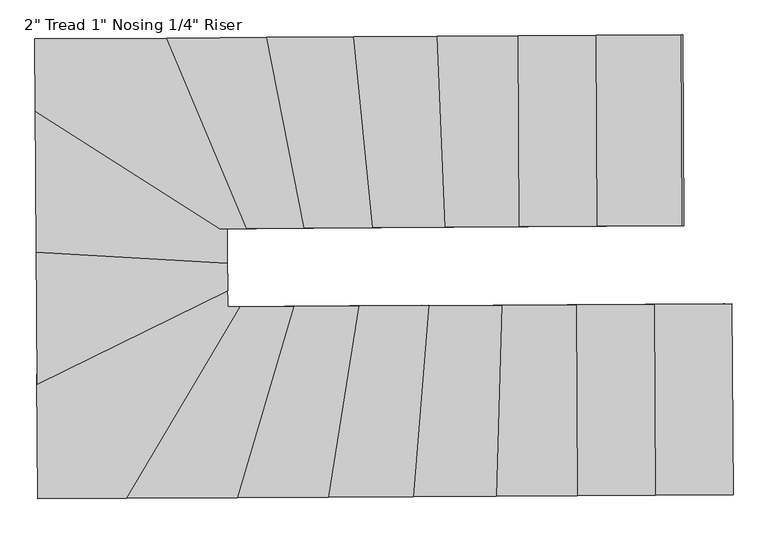
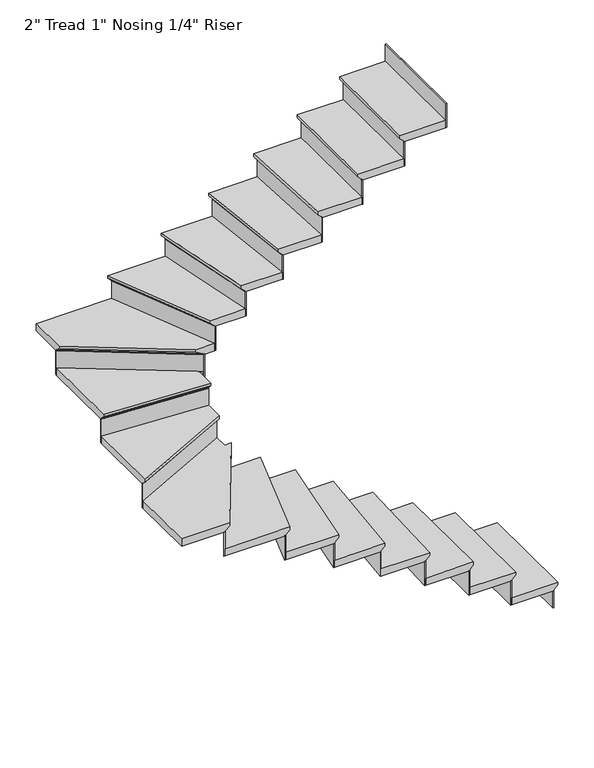
"""IFC4 building model written with IfcOpenShell, lengths in millimetres: stair flight geometry."""

from ifc_helpers import new_model, si_unit, origin, place, context, project, spatial, faceted_brep, source, transform, mapped, element, save


def stair_flight_20cd7bae(model_context):
    return source(origin(), model_context, "Body", "Brep", [
        faceted_brep([(-120.6930289, -3539.621908, 3350.6833333), (-120.6930289, -3539.621908, 3369.7333333), (-116.4891496, -4225.4090232, 3369.7333333), (-116.4891496, -4225.4090232, 3350.6833333), (-146.0925517, -3539.7776072, 3325.2833333), (-141.8886723, -4225.5647224, 3325.2833333), (-425.4873024, -3541.4902988, 3369.7333333), (-421.283423, -4227.277414, 3369.7333333), (-141.8886723, -4225.5647224, 3318.9333333), (-421.283423, -4227.277414, 3318.9333333), (-425.4873024, -3541.4902988, 3318.9333333), (-146.0925517, -3539.7776072, 3318.9333333)], [[[0, 1, 2, 3]], [[4, 0, 3, 5]], [[2, 1, 6, 7]], [[8, 9, 10, 11]], [[2, 7, 9, 8, 5, 3]], [[8, 11, 4, 5]], [[6, 1, 0, 4, 11, 10]], [[7, 6, 10, 9]]]),
        faceted_brep([(-146.0925517, -3539.7776072, 3318.9333333), (-146.0925517, -3539.7776072, 3200.4), (-152.4424324, -3539.816532, 3200.4), (-152.4424324, -3539.816532, 3318.9333333), (-141.8886723, -4225.5647224, 3318.9333333), (-148.238553, -4225.6036472, 3318.9333333), (-148.238553, -4225.6036472, 3200.4), (-141.8886723, -4225.5647224, 3200.4)], [[[0, 1, 2, 3]], [[4, 5, 6, 7]], [[1, 0, 4, 7]], [[2, 1, 7, 6]], [[3, 2, 6, 5]], [[0, 3, 5, 4]]]),
        faceted_brep([(-425.4873024, -3541.4902988, 3488.2666667), (-425.4873024, -3541.4902988, 3318.9333333), (-431.8371831, -3541.5292236, 3318.9333333), (-431.8371831, -3541.5292236, 3488.2666667), (-421.283423, -4227.277414, 3488.2666667), (-427.6333037, -4227.3163388, 3488.2666667), (-427.6333037, -4227.3163388, 3318.9333333), (-421.283423, -4227.277414, 3318.9333333)], [[[0, 1, 2, 3]], [[4, 5, 6, 7]], [[1, 0, 4, 7]], [[2, 1, 7, 6]], [[3, 2, 6, 5]], [[0, 3, 5, 4]]]),
        faceted_brep([(-395.8839002, -4227.1217148, 3539.0666667), (-400.0877796, -3541.3345996, 3539.0666667), (-704.882053, -3543.2029904, 3539.0666667), (-700.6781736, -4228.9901056, 3539.0666667), (-421.283423, -4227.277414, 3488.2666667), (-700.6781736, -4228.9901056, 3488.2666667), (-704.882053, -3543.2029904, 3488.2666667), (-425.4873024, -3541.4902988, 3488.2666667), (-421.283423, -4227.277414, 3494.6166667), (-395.8839002, -4227.1217148, 3520.0166667), (-425.4873024, -3541.4902988, 3494.6166667), (-400.0877796, -3541.3345996, 3520.0166667)], [[[0, 1, 2, 3]], [[4, 5, 6, 7]], [[0, 3, 5, 4, 8, 9]], [[4, 7, 10, 8]], [[2, 1, 11, 10, 7, 6]], [[3, 2, 6, 5]], [[11, 1, 0, 9]], [[10, 11, 9, 8]]]),
        faceted_brep([(-704.882053, -3543.2029904, 3657.6), (-704.882053, -3543.2029904, 3488.2666667), (-711.2319337, -3543.2419152, 3488.2666667), (-711.2319337, -3543.2419152, 3657.6), (-700.6781736, -4228.9901056, 3657.6), (-707.0280543, -4229.0290304, 3657.6), (-707.0280543, -4229.0290304, 3488.2666667), (-700.6781736, -4228.9901056, 3488.2666667)], [[[0, 1, 2, 3]], [[4, 5, 6, 7]], [[1, 0, 4, 7]], [[2, 1, 7, 6]], [[3, 2, 6, 5]], [[0, 3, 5, 4]]]),
        faceted_brep([(-675.2786508, -4228.8344064, 3708.4), (-679.4825302, -3543.0472912, 3708.4), (-971.9344004, -3544.840023, 3708.4), (-992.4483132, -4230.7786584, 3708.4), (-700.6781736, -4228.9901056, 3657.6), (-992.4483132, -4230.7786584, 3657.6), (-971.9344004, -3544.840023, 3657.6), (-704.882053, -3543.2029904, 3657.6), (-700.6781736, -4228.9901056, 3663.95), (-675.2786508, -4228.8344064, 3689.35), (-704.882053, -3543.2029904, 3663.95), (-679.4825302, -3543.0472912, 3689.35)], [[[0, 1, 2, 3]], [[4, 5, 6, 7]], [[0, 3, 5, 4, 8, 9]], [[4, 7, 10, 8]], [[2, 1, 11, 10, 7, 6]], [[3, 2, 6, 5]], [[11, 1, 0, 9]], [[10, 11, 9, 8]]]),
        faceted_brep([(-971.9344004, -3544.840023, 3826.9333333), (-971.9344004, -3544.840023, 3657.6), (-978.2884043, -3544.8789731, 3657.6), (-978.2884043, -3544.8789731, 3826.9333333), (-992.4483132, -4230.7786584, 3826.9333333), (-998.8023171, -4230.8176085, 3826.9333333), (-998.8023171, -4230.8176085, 3657.6), (-992.4483132, -4230.7786584, 3657.6)], [[[0, 1, 2, 3]], [[4, 5, 6, 7]], [[1, 0, 4, 7]], [[2, 1, 7, 6]], [[3, 2, 6, 5]], [[0, 3, 5, 4]]]),
        faceted_brep([(-967.0322975, -4230.6228581, 3877.7333333), (-946.5183848, -3544.6842227, 3877.7333333), (-1233.842238, -3546.4455197, 3877.7333333), (-1289.4900883, -4232.5995264, 3877.7333333), (-992.4483132, -4230.7786584, 3826.9333333), (-1289.4900883, -4232.5995264, 3826.9333333), (-1233.842238, -3546.4455197, 3826.9333333), (-971.9344004, -3544.840023, 3826.9333333), (-992.4483132, -4230.7786584, 3833.2833333), (-967.0322975, -4230.6228581, 3858.6833333), (-971.9344004, -3544.840023, 3833.2833333), (-946.5183848, -3544.6842227, 3858.6833333)], [[[0, 1, 2, 3]], [[4, 5, 6, 7]], [[0, 3, 5, 4, 8, 9]], [[4, 7, 10, 8]], [[2, 1, 11, 10, 7, 6]], [[3, 2, 6, 5]], [[11, 1, 0, 9]], [[10, 11, 9, 8]]]),
        faceted_brep([(-1233.842238, -3546.4455197, 3996.2666667), (-1233.842238, -3546.4455197, 3826.9333333), (-1240.2162558, -3546.4845925, 3826.9333333), (-1240.2162558, -3546.4845925, 3996.2666667), (-1289.4900883, -4232.5995264, 3996.2666667), (-1295.8641061, -4232.6385992, 3996.2666667), (-1295.8641061, -4232.6385992, 3826.9333333), (-1289.4900883, -4232.5995264, 3826.9333333)], [[[0, 1, 2, 3]], [[4, 5, 6, 7]], [[1, 0, 4, 7]], [[2, 1, 7, 6]], [[3, 2, 6, 5]], [[0, 3, 5, 4]]]),
        faceted_brep([(-1263.994017, -4232.4432353, 4047.0666667), (-1208.3461666, -3546.2892286, 4047.0666667), (-1486.5415383, -3547.994568, 4047.0666667), (-1596.081167, -4234.4789317, 4047.0666667), (-1289.4900883, -4232.5995264, 3996.2666667), (-1596.081167, -4234.4789317, 3996.2666667), (-1486.5415383, -3547.994568, 3996.2666667), (-1233.842238, -3546.4455197, 3996.2666667), (-1289.4900883, -4232.5995264, 4002.6166667), (-1263.994017, -4232.4432353, 4028.0166667), (-1233.842238, -3546.4455197, 4002.6166667), (-1208.3461666, -3546.2892286, 4028.0166667)], [[[0, 1, 2, 3]], [[4, 5, 6, 7]], [[0, 3, 5, 4, 8, 9]], [[4, 7, 10, 8]], [[2, 1, 11, 10, 7, 6]], [[3, 2, 6, 5]], [[11, 1, 0, 9]], [[10, 11, 9, 8]]]),
        faceted_brep([(-1486.5415383, -3547.994568, 4165.6), (-1486.5415383, -3547.994568, 3996.2666667), (-1492.9781659, -3548.0340246, 3996.2666667), (-1492.9781659, -3548.0340246, 4165.6), (-1596.081167, -4234.4789317, 4165.6), (-1602.5177946, -4234.5183882, 4165.6), (-1602.5177946, -4234.5183882, 3996.2666667), (-1596.081167, -4234.4789317, 3996.2666667)], [[[0, 1, 2, 3]], [[4, 5, 6, 7]], [[1, 0, 4, 7]], [[2, 1, 7, 6]], [[3, 2, 6, 5]], [[0, 3, 5, 4]]]),
        faceted_brep([(-1570.3346568, -4234.3211054, 4216.4), (-1460.7950281, -3547.8367418, 4216.4), (-1720.1488607, -3549.4265824, 4216.4), (-1922.8306159, -4236.4819079, 4216.4), (-1596.081167, -4234.4789317, 4165.6), (-1922.8306159, -4236.4819079, 4165.6), (-1720.1488607, -3549.4265824, 4165.6), (-1486.5415383, -3547.994568, 4165.6), (-1596.081167, -4234.4789317, 4171.95), (-1570.3346568, -4234.3211054, 4197.35), (-1486.5415383, -3547.994568, 4171.95), (-1460.7950281, -3547.8367418, 4197.35)], [[[0, 1, 2, 3]], [[4, 5, 6, 7]], [[0, 3, 5, 4, 8, 9]], [[4, 7, 10, 8]], [[2, 1, 11, 10, 7, 6]], [[3, 2, 6, 5]], [[11, 1, 0, 9]], [[10, 11, 9, 8]]]),
        faceted_brep([(-1720.1488607, -3549.4265824, 4334.9333333), (-1720.1488607, -3549.4265824, 4165.6), (-1726.781397, -3549.4672399, 4165.6), (-1726.781397, -3549.4672399, 4334.9333333), (-1922.8306159, -4236.4819079, 4334.9333333), (-1929.4631522, -4236.5225654, 4334.9333333), (-1929.4631522, -4236.5225654, 4165.6), (-1922.8306159, -4236.4819079, 4165.6)], [[[0, 1, 2, 3]], [[4, 5, 6, 7]], [[1, 0, 4, 7]], [[2, 1, 7, 6]], [[3, 2, 6, 5]], [[0, 3, 5, 4]]]),
        faceted_brep([(-1896.3004707, -4236.3192779, 4385.7333333), (-1693.6187155, -3549.2639524, 4385.7333333), (-1917.3665941, -3550.6355283, 4385.7333333), (-2324.8688668, -4238.9464049, 4385.7333333), (-1922.8306159, -4236.4819079, 4334.9333333), (-2324.8688668, -4238.9464049, 4334.9333333), (-1917.3665941, -3550.6355283, 4334.9333333), (-1720.1488607, -3549.4265824, 4334.9333333), (-1922.8306159, -4236.4819079, 4341.2833333), (-1896.3004707, -4236.3192779, 4366.6833333), (-1720.1488607, -3549.4265824, 4341.2833333), (-1693.6187155, -3549.2639524, 4366.6833333)], [[[0, 1, 2, 3]], [[4, 5, 6, 7]], [[0, 3, 5, 4, 8, 9]], [[4, 7, 10, 8]], [[2, 1, 11, 10, 7, 6]], [[3, 2, 6, 5]], [[11, 1, 0, 9]], [[10, 11, 9, 8]]]),
        faceted_brep([(-1917.3665941, -3550.6355283, 4504.2666667), (-1917.3665941, -3550.6355283, 4334.9333333), (-1924.7728783, -3550.6809289, 4334.9333333), (-1924.7728783, -3550.6809289, 4504.2666667), (-2324.8688668, -4238.9464049, 4504.2666667), (-2332.275151, -4238.9918055, 4504.2666667), (-2332.275151, -4238.9918055, 4334.9333333), (-2324.8688668, -4238.9464049, 4334.9333333)], [[[0, 1, 2, 3]], [[4, 5, 6, 7]], [[1, 0, 4, 7]], [[2, 1, 7, 6]], [[3, 2, 6, 5]], [[0, 3, 5, 4]]]),
        faceted_brep([(-2615.3480869, -3801.2875551, 4555.0666667), (-2612.6544213, -4240.7105322, 4555.0666667), (-2295.24373, -4238.7648026, 4555.0666667), (-1887.7414574, -3550.4539261, 4555.0666667), (-1931.0711854, -3550.7195376, 4555.0666667), (-1931.5966592, -3464.9979706, 4555.0666667), (-2612.6544213, -4240.7105322, 4504.2666667), (-2615.3480869, -3801.2875551, 4504.2666667), (-1931.5966592, -3464.9979706, 4504.2666667), (-1931.0711854, -3550.7195376, 4504.2666667), (-1917.3665941, -3550.6355283, 4504.2666667), (-2324.8688668, -4238.9464049, 4504.2666667), (-1917.3665941, -3550.6355283, 4510.6166667), (-2324.8688668, -4238.9464049, 4510.6166667), (-1887.7414574, -3550.4539261, 4536.0166667), (-2295.24373, -4238.7648026, 4536.0166667)], [[[0, 1, 2, 3, 4, 5]], [[6, 7, 8, 9, 10, 11]], [[1, 0, 7, 6]], [[11, 10, 12, 13]], [[5, 4, 9, 8]], [[0, 5, 8, 7]], [[14, 3, 2, 15]], [[12, 14, 15, 13]], [[4, 3, 14, 12, 10, 9]], [[2, 1, 6, 11, 13, 15]]]),
        faceted_brep([(-1931.5966592, -3464.9979706, 4673.6), (-1931.5966592, -3464.9979706, 4504.2666667), (-1931.6399076, -3457.9427742, 4504.2666667), (-1931.6399076, -3457.9427742, 4673.6), (-2615.3480869, -3801.2875551, 4673.6), (-2615.3913353, -3794.2323587, 4673.6), (-2615.3913353, -3794.2323587, 4504.2666667), (-2615.3480869, -3801.2875551, 4504.2666667)], [[[0, 1, 2, 3]], [[4, 5, 6, 7]], [[1, 0, 4, 7]], [[2, 1, 7, 6]], [[3, 2, 6, 5]], [[0, 3, 5, 4]]]),
        faceted_brep([(-2615.1750933, -3829.5083406, 4724.4), (-1931.4236656, -3493.2187561, 4724.4), (-1932.1828972, -3369.3638122, 4724.4), (-2618.2387587, -3329.7265819, 4724.4), (-2615.3480869, -3801.2875551, 4673.6), (-2618.2387587, -3329.7265819, 4673.6), (-1932.1828972, -3369.3638122, 4673.6), (-1931.5966592, -3464.9979706, 4673.6), (-2615.3480869, -3801.2875551, 4679.95), (-2615.1750933, -3829.5083406, 4705.35), (-1931.5966592, -3464.9979706, 4679.95), (-1931.4236656, -3493.2187561, 4705.35)], [[[0, 1, 2, 3]], [[4, 5, 6, 7]], [[0, 3, 5, 4, 8, 9]], [[4, 7, 10, 8]], [[2, 1, 11, 10, 7, 6]], [[3, 2, 6, 5]], [[11, 1, 0, 9]], [[10, 11, 9, 8]]]),
        faceted_brep([(-1932.1828972, -3369.3638122, 4842.9333333), (-1932.1828972, -3369.3638122, 4673.6), (-1932.2219015, -3363.0009693, 4673.6), (-1932.2219015, -3363.0009693, 4842.9333333), (-2618.2387587, -3329.7265819, 4842.9333333), (-2618.277763, -3323.363739, 4842.9333333), (-2618.277763, -3323.363739, 4673.6), (-2618.2387587, -3329.7265819, 4673.6)], [[[0, 1, 2, 3]], [[4, 5, 6, 7]], [[1, 0, 4, 7]], [[2, 1, 7, 6]], [[3, 2, 6, 5]], [[0, 3, 5, 4]]]),
        faceted_brep([(-2618.0827416, -3355.1779533, 4893.7333333), (-1932.0268801, -3394.8151835, 4893.7333333), (-1932.783877, -3271.3247869, 4893.7333333), (-1912.0496222, -3271.1976858, 4893.7333333), (-2621.364296, -2819.8515342, 4893.7333333), (-2618.2387587, -3329.7265819, 4842.9333333), (-2621.364296, -2819.8515342, 4842.9333333), (-1912.0496222, -3271.1976858, 4842.9333333), (-1932.783877, -3271.3247869, 4842.9333333), (-1932.1828972, -3369.3638122, 4842.9333333), (-2618.2387587, -3329.7265819, 4849.2833333), (-2618.0827416, -3355.1779533, 4874.6833333), (-1932.1828972, -3369.3638122, 4849.2833333), (-1932.0268801, -3394.8151835, 4874.6833333)], [[[0, 1, 2, 3, 4]], [[5, 6, 7, 8, 9]], [[0, 4, 6, 5, 10, 11]], [[5, 9, 12, 10]], [[2, 1, 13, 12, 9, 8]], [[3, 2, 8, 7]], [[4, 3, 7, 6]], [[13, 1, 0, 11]], [[12, 13, 11, 10]]]),
        faceted_brep([(-1912.0496222, -3271.1976858, 5012.2666667), (-1912.0496222, -3271.1976858, 4842.9333333), (-1900.3341194, -3271.1258697, 4842.9333333), (-1900.3341194, -3271.1258697, 5012.2666667), (-2621.364296, -2819.8515342, 5012.2666667), (-2621.4106144, -2812.2955182, 5012.2666667), (-2621.4106144, -2812.2955182, 4842.9333333), (-2621.364296, -2819.8515342, 4842.9333333)], [[[0, 1, 2, 3]], [[4, 5, 6, 7]], [[1, 0, 4, 7]], [[2, 1, 7, 6]], [[3, 2, 6, 5]], [[0, 3, 5, 4]]]),
        faceted_brep([(-2121.4312205, -2586.6683113, 5063.0666667), (-2622.7748716, -2589.7415511, 5063.0666667), (-2621.1790223, -2850.0755978, 5063.0666667), (-1958.9116334, -3271.4849502, 5063.0666667), (-1835.3232791, -3270.7273529, 5063.0666667), (-2622.7748716, -2589.7415511, 5012.2666667), (-2121.4312205, -2586.6683113, 5012.2666667), (-1835.3232791, -3270.7273529, 5012.2666667), (-1912.0496222, -3271.1976858, 5012.2666667), (-2621.364296, -2819.8515342, 5012.2666667), (-2621.364296, -2819.8515342, 5018.6166667), (-2621.1790223, -2850.0755978, 5044.0166667), (-1912.0496222, -3271.1976858, 5018.6166667), (-1958.9116334, -3271.4849502, 5044.0166667)], [[[0, 1, 2, 3, 4]], [[5, 6, 7, 8, 9]], [[1, 0, 6, 5]], [[2, 1, 5, 9, 10, 11]], [[9, 8, 12, 10]], [[0, 4, 7, 6]], [[13, 3, 2, 11]], [[12, 13, 11, 10]], [[4, 3, 13, 12, 8, 7]]]),
        faceted_brep([(-1835.3232791, -3270.7273529, 5181.6), (-1835.3232791, -3270.7273529, 5012.2666667), (-1828.4578405, -3270.6852677, 5012.2666667), (-1828.4578405, -3270.6852677, 5181.6), (-2121.4312205, -2586.6683113, 5181.6), (-2114.5657819, -2586.6262261, 5181.6), (-2114.5657819, -2586.6262261, 5012.2666667), (-2121.4312205, -2586.6683113, 5012.2666667)], [[[0, 1, 2, 3]], [[4, 5, 6, 7]], [[1, 0, 4, 7]], [[2, 1, 7, 6]], [[3, 2, 6, 5]], [[0, 3, 5, 4]]]),
        faceted_brep([(-2148.8929752, -2586.8366521, 5232.4), (-1862.7850338, -3270.8956936, 5232.4), (-1630.6514822, -3269.4727134, 5232.4), (-1765.0751589, -2584.4838464, 5232.4), (-2121.4312205, -2586.6683113, 5181.6), (-1765.0751589, -2584.4838464, 5181.6), (-1630.6514822, -3269.4727134, 5181.6), (-1835.3232791, -3270.7273529, 5181.6), (-2121.4312205, -2586.6683113, 5187.95), (-2148.8929752, -2586.8366521, 5213.35), (-1835.3232791, -3270.7273529, 5187.95), (-1862.7850338, -3270.8956936, 5213.35)], [[[0, 1, 2, 3]], [[4, 5, 6, 7]], [[0, 3, 5, 4, 8, 9]], [[4, 7, 10, 8]], [[2, 1, 11, 10, 7, 6]], [[3, 2, 6, 5]], [[11, 1, 0, 9]], [[10, 11, 9, 8]]]),
        faceted_brep([(-1630.6514822, -3269.4727134, 5350.9333333), (-1630.6514822, -3269.4727134, 5181.6), (-1624.1881401, -3269.4330931, 5181.6), (-1624.1881401, -3269.4330931, 5350.9333333), (-1765.0751589, -2584.4838464, 5350.9333333), (-1758.6118168, -2584.4442261, 5350.9333333), (-1758.6118168, -2584.4442261, 5181.6), (-1765.0751589, -2584.4838464, 5181.6)], [[[0, 1, 2, 3]], [[4, 5, 6, 7]], [[1, 0, 4, 7]], [[2, 1, 7, 6]], [[3, 2, 6, 5]], [[0, 3, 5, 4]]]),
        faceted_brep([(-1790.9285273, -2584.6423277, 5401.7333333), (-1656.5048506, -3269.6311948, 5401.7333333), (-1385.319119, -3267.9688245, 5401.7333333), (-1452.3132293, -2582.5666138, 5401.7333333), (-1765.0751589, -2584.4838464, 5350.9333333), (-1452.3132293, -2582.5666138, 5350.9333333), (-1385.319119, -3267.9688245, 5350.9333333), (-1630.6514822, -3269.4727134, 5350.9333333), (-1765.0751589, -2584.4838464, 5357.2833333), (-1790.9285273, -2584.6423277, 5382.6833333), (-1630.6514822, -3269.4727134, 5357.2833333), (-1656.5048506, -3269.6311948, 5382.6833333)], [[[0, 1, 2, 3]], [[4, 5, 6, 7]], [[0, 3, 5, 4, 8, 9]], [[4, 7, 10, 8]], [[2, 1, 11, 10, 7, 6]], [[3, 2, 6, 5]], [[11, 1, 0, 9]], [[10, 11, 9, 8]]]),
        faceted_brep([(-1385.319119, -3267.9688245, 5520.2666667), (-1385.319119, -3267.9688245, 5350.9333333), (-1378.942678, -3267.9297369, 5350.9333333), (-1378.942678, -3267.9297369, 5520.2666667), (-1452.3132293, -2582.5666138, 5520.2666667), (-1445.9367882, -2582.5275262, 5520.2666667), (-1445.9367882, -2582.5275262, 5350.9333333), (-1452.3132293, -2582.5666138, 5350.9333333)], [[[0, 1, 2, 3]], [[4, 5, 6, 7]], [[1, 0, 4, 7]], [[2, 1, 7, 6]], [[3, 2, 6, 5]], [[0, 3, 5, 4]]]),
        faceted_brep([(-1477.8189934, -2582.7229643, 5571.0666667), (-1410.8248832, -3268.125175, 5571.0666667), (-1125.1141805, -3266.3737666, 5571.0666667), (-1153.9085026, -2580.7373909, 5571.0666667), (-1452.3132293, -2582.5666138, 5520.2666667), (-1153.9085026, -2580.7373909, 5520.2666667), (-1125.1141805, -3266.3737666, 5520.2666667), (-1385.319119, -3267.9688245, 5520.2666667), (-1452.3132293, -2582.5666138, 5526.6166667), (-1477.8189934, -2582.7229643, 5552.0166667), (-1385.319119, -3267.9688245, 5526.6166667), (-1410.8248832, -3268.125175, 5552.0166667)], [[[0, 1, 2, 3]], [[4, 5, 6, 7]], [[0, 3, 5, 4, 8, 9]], [[4, 7, 10, 8]], [[2, 1, 11, 10, 7, 6]], [[3, 2, 6, 5]], [[11, 1, 0, 9]], [[10, 11, 9, 8]]]),
        faceted_brep([(-1125.1141805, -3266.3737666, 5689.6), (-1125.1141805, -3266.3737666, 5520.2666667), (-1118.7602189, -3266.3348167, 5520.2666667), (-1118.7602189, -3266.3348167, 5689.6), (-1153.9085026, -2580.7373909, 5689.6), (-1147.554541, -2580.6984411, 5689.6), (-1147.554541, -2580.6984411, 5520.2666667), (-1153.9085026, -2580.7373909, 5520.2666667)], [[[0, 1, 2, 3]], [[4, 5, 6, 7]], [[1, 0, 4, 7]], [[2, 1, 7, 6]], [[3, 2, 6, 5]], [[0, 3, 5, 4]]]),
        faceted_brep([(-1179.3243487, -2580.8931902, 5740.4), (-1150.5300267, -3266.5295659, 5740.4), (-858.0309746, -3264.7365448, 5740.4), (-862.2348539, -2578.9494296, 5740.4), (-1153.9085026, -2580.7373909, 5689.6), (-862.2348539, -2578.9494296, 5689.6), (-858.0309746, -3264.7365448, 5689.6), (-1125.1141805, -3266.3737666, 5689.6), (-1153.9085026, -2580.7373909, 5695.95), (-1179.3243487, -2580.8931902, 5721.35), (-1125.1141805, -3266.3737666, 5695.95), (-1150.5300267, -3266.5295659, 5721.35)], [[[0, 1, 2, 3]], [[4, 5, 6, 7]], [[0, 3, 5, 4, 8, 9]], [[4, 7, 10, 8]], [[2, 1, 11, 10, 7, 6]], [[3, 2, 6, 5]], [[11, 1, 0, 9]], [[10, 11, 9, 8]]]),
        faceted_brep([(-858.0309746, -3264.7365448, 5858.9333333), (-858.0309746, -3264.7365448, 5689.6), (-851.6810939, -3264.69762, 5689.6), (-851.6810939, -3264.69762, 5858.9333333), (-862.2348539, -2578.9494296, 5858.9333333), (-855.8849733, -2578.9105048, 5858.9333333), (-855.8849733, -2578.9105048, 5689.6), (-862.2348539, -2578.9494296, 5689.6)], [[[0, 1, 2, 3]], [[4, 5, 6, 7]], [[1, 0, 4, 7]], [[2, 1, 7, 6]], [[3, 2, 6, 5]], [[0, 3, 5, 4]]]),
        faceted_brep([(-887.6343767, -2579.1051288, 5909.7333333), (-883.4304974, -3264.8922441, 5909.7333333), (-578.6362239, -3263.0238532, 5909.7333333), (-582.8401033, -2577.236738, 5909.7333333), (-862.2348539, -2578.9494296, 5858.9333333), (-582.8401033, -2577.236738, 5858.9333333), (-578.6362239, -3263.0238532, 5858.9333333), (-858.0309746, -3264.7365448, 5858.9333333), (-862.2348539, -2578.9494296, 5865.2833333), (-887.6343767, -2579.1051288, 5890.6833333), (-858.0309746, -3264.7365448, 5865.2833333), (-883.4304974, -3264.8922441, 5890.6833333)], [[[0, 1, 2, 3]], [[4, 5, 6, 7]], [[0, 3, 5, 4, 8, 9]], [[4, 7, 10, 8]], [[2, 1, 11, 10, 7, 6]], [[3, 2, 6, 5]], [[11, 1, 0, 9]], [[10, 11, 9, 8]]]),
        faceted_brep([(-578.6362239, -3263.0238532, 6028.2666667), (-578.6362239, -3263.0238532, 5858.9333333), (-572.2863432, -3262.9849284, 5858.9333333), (-572.2863432, -3262.9849284, 6028.2666667), (-582.8401033, -2577.236738, 6028.2666667), (-576.4902226, -2577.1978132, 6028.2666667), (-576.4902226, -2577.1978132, 5858.9333333), (-582.8401033, -2577.236738, 5858.9333333)], [[[0, 1, 2, 3]], [[4, 5, 6, 7]], [[1, 0, 4, 7]], [[2, 1, 7, 6]], [[3, 2, 6, 5]], [[0, 3, 5, 4]]]),
        faceted_brep([(-299.2414733, -3261.3111616, 6197.6), (-299.2414733, -3261.3111616, 6028.2666667), (-292.8915926, -3261.2722368, 6028.2666667), (-292.8915926, -3261.2722368, 6197.6), (-303.4453527, -2575.5240464, 6197.6), (-297.095472, -2575.4851216, 6197.6), (-297.095472, -2575.4851216, 6028.2666667), (-303.4453527, -2575.5240464, 6028.2666667)], [[[0, 1, 2, 3]], [[4, 5, 6, 7]], [[1, 0, 4, 7]], [[2, 1, 7, 6]], [[3, 2, 6, 5]], [[0, 3, 5, 4]]]),
        faceted_brep([(-608.2396261, -2577.3924372, 6079.0666667), (-604.0357467, -3263.1795525, 6079.0666667), (-299.2414733, -3261.3111616, 6079.0666667), (-303.4453527, -2575.5240464, 6079.0666667), (-582.8401033, -2577.236738, 6028.2666667), (-303.4453527, -2575.5240464, 6028.2666667), (-299.2414733, -3261.3111616, 6028.2666667), (-578.6362239, -3263.0238532, 6028.2666667), (-582.8401033, -2577.236738, 6034.6166667), (-608.2396261, -2577.3924372, 6060.0166667), (-578.6362239, -3263.0238532, 6034.6166667), (-604.0357467, -3263.1795525, 6060.0166667)], [[[0, 1, 2, 3]], [[4, 5, 6, 7]], [[0, 3, 5, 4, 8, 9]], [[4, 7, 10, 8]], [[2, 1, 11, 10, 7, 6]], [[3, 2, 6, 5]], [[11, 1, 0, 9]], [[10, 11, 9, 8]]]),
    ])


if __name__ == "__main__":
    model = new_model("IFC4")
    model_context = context("Model", 3, world=origin())
    ifc_project = project(units=[si_unit("LENGTHUNIT", "METRE", prefix="MILLI")], contexts=[model_context])
    site = spatial("IfcSite", under=ifc_project)
    building = spatial("IfcBuilding", under=site)
    placement = place(None, origin())
    stair_flight_shape = stair_flight_20cd7bae(model_context)
    element("IfcStairFlight", 1, ObjectType="2\" Tread 1\" Nosing 1/4\" Riser", at=placement, inside=building, context=model_context, shape_type="MappedRepresentation", body=[
        mapped(stair_flight_shape, transform((0.0, 0.0, 0.0), x_axis=(1.0, 0.0, 0.0), y_axis=(0.0, 1.0, 0.0), z_axis=(0.0, 0.0, 1.0))),
    ])
    save(model, "model.ifc")
